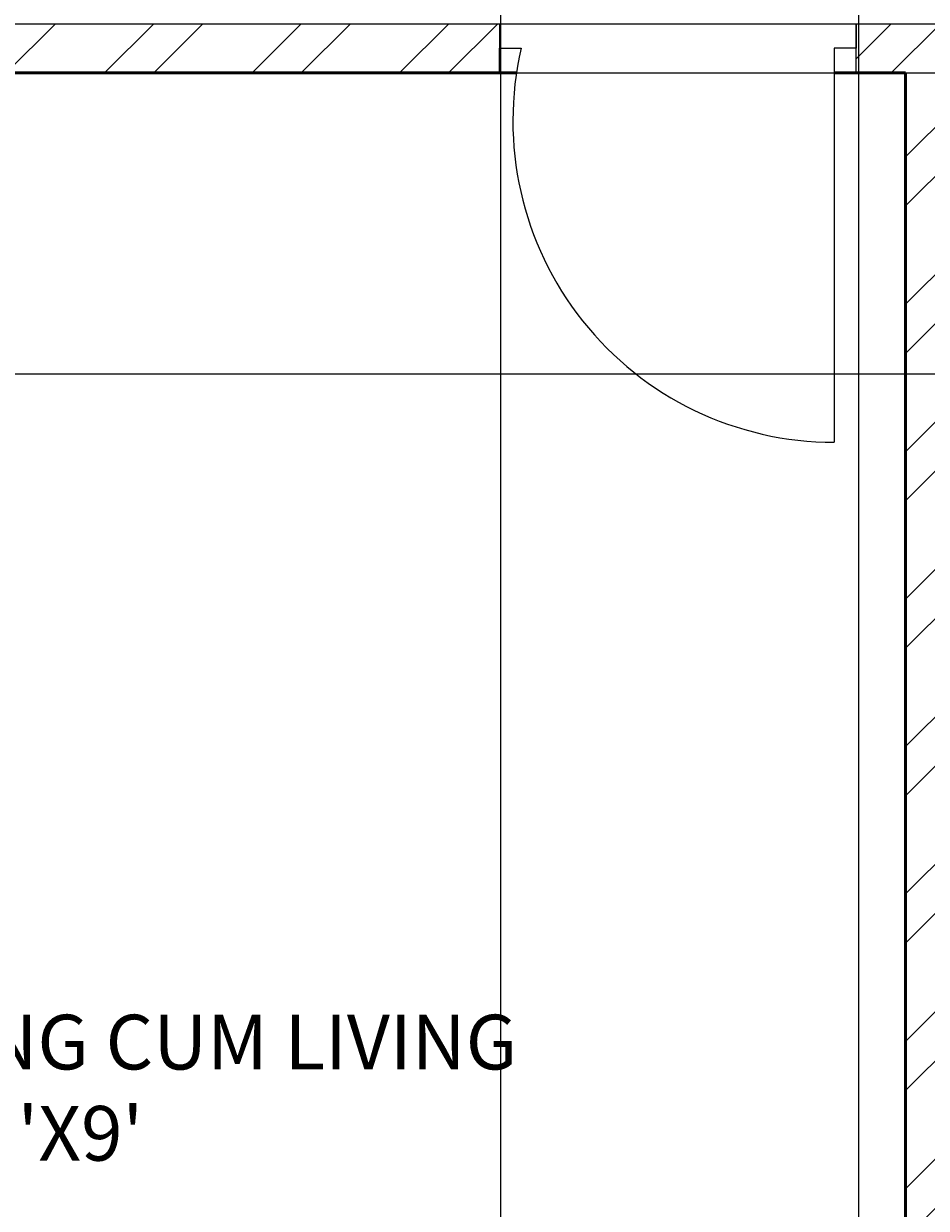
# Model space of a CAD drawing. Units: inches. Extents: x 2310 to 2937, y 1113 to 2410.
# Tile 7 of 23: x 2526 to 2609, y 1891 to 2000. Entities that reach past the tile are written whole.
import ezdxf

# ---------------------------------------------------------------- set-up
doc = ezdxf.new("R2010")
doc.units = ezdxf.units.IN
for name, color, linetype, lineweight in [('A-ANNO-DIMS', 2, 'Continuous', 18), ('A-AREA-IDEN', 7, 'Continuous', 18), ('A-DOOR', 31, 'Continuous', 25), ('A-WALL', 7, 'Continuous', 50), ('A-WALL-PATT', 85, 'Continuous', 13)]:
    doc.layers.add(name, color=color, linetype=linetype, lineweight=lineweight)
doc.styles.get("Standard").update_dxf_attribs({"font": 'arial.ttf'})
doc.dimstyles.get("Standard").update_dxf_attribs({"dimtxt": 0.18, "dimasz": 0.18, "dimexe": 0.18, "dimexo": 0.0625, "dimgap": 0.09, "dimtad": 0, "dimtih": 1, "dimtoh": 1, "dimdec": 4, "dimzin": 0, "dimdsep": 46, "dimtxsty": 'Standard', "dimcen": 0.09, "dimadec": 0, "dimazin": 0, "dimtfac": 1, "dimtdec": 4, "dimtofl": 0, "dimtmove": 0, "dimatfit": 3, "dimfxl": 1, "dimtolj": 1, "dimtzin": 0, "dimarcsym": 0})

# ---------------------------------------------------------------- blocks, each defined once
blk = doc.blocks.new('*D57')
at = {"layer": 'A-ANNO-DIMS', "color": 0, "lineweight": -2, "transparency": 16777216}
for p, q in [((2403.55, 1995.01), (2858.02, 1995.01)), ((2857.84, 1994.83), (2857.84, 1981.45)), ((2857.84, 1967.7), (2857.84, 1981.09)), ((2403.55, 1967.52), (2858.02, 1967.52))]:
    blk.add_line(p, q, dxfattribs=at)
at = {"layer": 'A-ANNO-DIMS', "color": 0, "transparency": 16777216}
for points in [[(2857.81, 1994.83), (2857.87, 1994.83), (2857.84, 1995.01)], [(2857.81, 1967.7), (2857.87, 1967.7), (2857.84, 1967.52)]]:
    blk.add_solid(points, dxfattribs=at)
at = {"layer": 'Defpoints', "color": 0, "transparency": 16777216}
for p in [(2403.49, 1995.01), (2403.49, 1967.52), (2857.84, 1967.52)]:
    blk.add_point(p, dxfattribs=at)
at = {"layer": 'A-ANNO-DIMS', "color": 0, "transparency": 16777216, "insert": (2857.84, 1981.27), "char_height": 0.18, "attachment_point": 5}
blk.add_mtext('\\A1;27.49', dxfattribs=at)
blk = doc.blocks.new('*D62')
at = {"layer": 'A-ANNO-DIMS', "color": 0, "lineweight": -2, "transparency": 16777216}
for p, q in [((2569.99, 2093.45), (2569.99, 1649.5)), ((2602.69, 2093.45), (2602.69, 1649.5)), ((2570.17, 1649.68), (2586.02, 1649.68)), ((2602.51, 1649.68), (2586.66, 1649.68))]:
    blk.add_line(p, q, dxfattribs=at)
at = {"layer": 'A-ANNO-DIMS', "color": 0, "transparency": 16777216}
for points in [[(2570.17, 1649.71), (2570.17, 1649.65), (2569.99, 1649.68)], [(2602.51, 1649.71), (2602.51, 1649.65), (2602.69, 1649.68)]]:
    blk.add_solid(points, dxfattribs=at)
at = {"layer": 'Defpoints', "color": 0, "transparency": 16777216}
for p in [(2569.99, 2093.51), (2602.69, 2093.51), (2602.69, 1649.68)]:
    blk.add_point(p, dxfattribs=at)
at = {"layer": 'A-ANNO-DIMS', "color": 0, "transparency": 16777216, "insert": (2586.34, 1649.68), "char_height": 0.18, "attachment_point": 5}
blk.add_mtext('\\A1;32.7', dxfattribs=at)
blk = doc.blocks.new('*D64')
at = {"layer": 'A-ANNO-DIMS', "color": 0, "lineweight": -2, "transparency": 16777216}
for p, q in [((2524.527191, 2046.513944), (2858.015941, 2046.513944)), ((2857.835941, 2046.333944), (2857.835941, 2023.193944)), ((2857.835941, 1999.693944), (2857.835941, 2022.833944)), ((2524.527191, 1999.513944), (2858.015941, 1999.513944))]:
    blk.add_line(p, q, dxfattribs=at)
at = {"layer": 'A-ANNO-DIMS', "color": 0, "transparency": 16777216}
for points in [[(2857.805941, 2046.333944), (2857.865941, 2046.333944), (2857.835941, 2046.513944)], [(2857.805941, 1999.693944), (2857.865941, 1999.693944), (2857.835941, 1999.513944)]]:
    blk.add_solid(points, dxfattribs=at)
at = {"layer": 'Defpoints', "color": 0, "transparency": 16777216}
for p in [(2524.464691, 2046.513944), (2857.835941, 2046.513944), (2524.464691, 1999.513944)]:
    blk.add_point(p, dxfattribs=at)
at = {"layer": 'A-ANNO-DIMS', "color": 0, "transparency": 16777216, "insert": (2857.835941, 2023.013944), "char_height": 0.18, "attachment_point": 5}
blk.add_mtext('\\A1;47', dxfattribs=at)

msp = doc.modelspace()

# ---------------------------------------------------------------- hatches: boundary and pattern name
at = {"layer": 'A-WALL-PATT'}
h = msp.add_hatch(dxfattribs=at)
h.set_pattern_fill('ANSI32', color=256)
h.paths.add_polyline_path([(2639.1394, 2356.5139), (2563.662, 2356.5139), (2563.662, 2347.5139), (2606.9859, 2347.5139), (2606.9859, 2210.5139), (2514.2692, 2210.5139), (2514.2692, 2206.0139), (2606.9859, 2206.0139), (2606.9859, 2098.0139), (2602.689, 2098.0139), (2602.689, 2093.5139), (2615.5262, 2093.5139), (2615.5262, 2095.7639), (2615.5262, 2098.0139), (2611.4859, 2098.0139), (2611.4859, 2206.0139), (2703.9391, 2206.0139), (2703.9391, 2208.2639), (2703.9391, 2210.5139), (2611.4859, 2210.5139), (2611.4859, 2347.5139), (2639.1394, 2347.5139)])
h.paths.add_polyline_path([(2823.9859, 2356.5139), (2699.1394, 2356.5139), (2699.1394, 2347.5139), (2738.4859, 2347.5139), (2738.4859, 2343.9266), (2742.9859, 2343.9266), (2742.9859, 2347.5139), (2814.9859, 2347.5139), (2814.9859, 2336.76), (2823.9859, 2336.76)])
h.paths.add_polyline_path([(2823.9859, 2312.76), (2814.9859, 2312.76), (2814.9859, 2299.5139), (2742.9859, 2299.5139), (2742.9859, 2323.0159), (2740.7359, 2323.0159), (2738.4859, 2323.0159), (2738.4859, 2210.5139), (2734.5483, 2210.5139), (2734.5483, 2206.0139), (2746.8769, 2206.0139), (2746.8769, 2208.2639), (2746.8769, 2210.5139), (2742.9859, 2210.5139), (2742.9859, 2295.0139), (2814.9859, 2295.0139), (2814.9859, 2269.8977), (2823.9859, 2269.8977)])
h.paths.add_polyline_path([(2823.9859, 2210.5139), (2823.9859, 2233.8977), (2819.4859, 2233.8977), (2814.9859, 2233.8977), (2814.9859, 2210.5139), (2769.9745, 2210.5139), (2769.9745, 2206.0139), (2814.9859, 2206.0139), (2814.9859, 2178.3027), (2823.9859, 2178.3027)])
h.paths.add_polyline_path([(2823.9859, 2118.3027), (2819.4859, 2118.3027), (2814.9859, 2118.3027), (2814.9859, 2098.0139), (2647.0333, 2098.0139), (2647.0333, 2093.5139), (2814.9859, 2093.5139), (2814.9859, 1999.5139), (2650.6052, 1999.5139), (2650.6052, 1995.0139), (2814.9859, 1995.0139), (2814.9859, 1969.9784), (2823.9859, 1969.9784)])
h.paths.add_polyline_path([(2403.4859, 2093.5139), (2569.9888, 2093.5139), (2569.9888, 2095.7639), (2569.9888, 2098.0139), (2403.4859, 2098.0139), (2403.4859, 2131.7587), (2394.4859, 2131.7587), (2394.4859, 1967.522), (2403.4859, 1967.522), (2403.4859, 1995.0139), (2569.8903, 1995.0139), (2569.8903, 1997.2639), (2569.8903, 1999.5139), (2403.4859, 1999.5139)])
h.paths.add_polyline_path([(2503.662, 2356.5139), (2394.4859, 2356.5139), (2394.4859, 2337.9231), (2398.9859, 2337.9231), (2403.4859, 2337.9231), (2403.4859, 2347.5139), (2475.4859, 2347.5139), (2475.4859, 2343.0384), (2479.9859, 2343.0384), (2479.9859, 2347.5139), (2503.662, 2347.5139)])
h.paths.add_polyline_path([(2498.3065, 1745.5139), (2479.9859, 1745.5139), (2479.9859, 1749.1663), (2477.7359, 1749.1663), (2475.4859, 1749.1663), (2475.4859, 1745.5139), (2403.4859, 1745.5139), (2403.4859, 1753.6409), (2398.9859, 1753.6409), (2394.4859, 1753.6409), (2394.4859, 1736.5139), (2498.3065, 1736.5139), (2498.3065, 1741.0139)])
h.paths.add_polyline_path([(2479.9859, 1882.5139), (2483.9367, 1882.5139), (2483.9367, 1887.0139), (2471.5501, 1887.0139), (2471.5501, 1885.1969), (2471.5501, 1882.5139), (2475.4859, 1882.5139), (2475.4859, 1798.0139), (2403.4859, 1798.0139), (2403.4859, 1828.0433), (2402.2852, 1828.0433), (2394.4859, 1828.0433), (2394.4859, 1777.6409), (2403.4859, 1777.6409), (2403.4859, 1793.5139), (2475.4859, 1793.5139), (2475.4859, 1769.1696), (2479.9859, 1769.1696)])
h.paths.add_polyline_path([(2403.4859, 1907.522), (2398.9859, 1907.522), (2394.4859, 1907.522), (2394.4859, 1864.0433), (2403.4859, 1864.0433), (2403.4859, 1882.5139), (2448.9325, 1882.5139), (2448.9325, 1884.7639), (2448.9325, 1887.0139), (2403.4859, 1887.0139)])
h.paths.add_polyline_path([(2702.2061, 1887.0139), (2611.4859, 1887.0139), (2611.4859, 1995.0139), (2615.6132, 1995.0139), (2615.6132, 1999.5139), (2602.4798, 1999.5139), (2602.4798, 1997.2639), (2602.4798, 1995.0139), (2606.9859, 1995.0139), (2606.9859, 1887.0139), (2516.2443, 1887.0139), (2516.2443, 1884.7639), (2516.2443, 1882.5139), (2606.9859, 1882.5139), (2606.9859, 1745.5139), (2558.3065, 1745.5139), (2558.3065, 1736.5139), (2638.8921, 1736.5139), (2638.8921, 1741.0139), (2638.8921, 1745.5139), (2611.4859, 1745.5139), (2611.4859, 1882.5139), (2702.2061, 1882.5139)])
h.paths.add_polyline_path([(2823.9859, 1909.9784), (2819.4859, 1909.9784), (2814.9859, 1909.9784), (2814.9859, 1887.0139), (2769.144, 1887.0139), (2769.144, 1884.7639), (2769.144, 1882.5139), (2814.9859, 1882.5139), (2814.9859, 1854.1704), (2823.9859, 1854.1704)])
h.paths.add_polyline_path([(2823.9859, 1818.1704), (2819.4859, 1818.1704), (2814.9859, 1818.1704), (2814.9859, 1798.0139), (2742.9859, 1798.0139), (2742.9859, 1882.5139), (2746.805, 1882.5139), (2746.805, 1887.0139), (2733.7334, 1887.0139), (2733.7334, 1884.7639), (2733.7334, 1882.5139), (2738.4859, 1882.5139), (2738.4859, 1771.1728), (2740.7359, 1771.1728), (2742.9859, 1771.1728), (2742.9859, 1793.5139), (2814.9859, 1793.5139), (2814.9859, 1783.6684), (2823.9859, 1783.6684)])
h.paths.add_polyline_path([(2823.9859, 1759.6684), (2814.9859, 1759.6684), (2814.9859, 1745.5139), (2742.9859, 1745.5139), (2742.9859, 1748.9831), (2740.7359, 1748.9831), (2738.4859, 1748.9831), (2738.4859, 1745.5139), (2698.8921, 1745.5139), (2698.8921, 1736.5139), (2823.9859, 1736.5139)])

# ---------------------------------------------------------------- linework, layer by layer
at = {"layer": 'A-DOOR'}
for p, q in [((2569.8903, 1999.5139), (2569.8903, 1995.0139)), ((2602.4798, 1995.0139), (2602.4798, 1999.5139)), ((2602.4798, 1999.5139), (2602.4798, 1997.2639)), ((2569.8903, 1995.0139), (2569.8903, 1997.2639)), ((2569.8903, 1997.2639), (2571.8903, 1997.2639)), ((2602.4798, 1997.2639), (2600.4798, 1997.2639)), ((2600.4798, 1997.2639), (2600.4798, 1961.2639))]:
    msp.add_line(p, q, dxfattribs=at)
msp.add_arc((2600.4798, 1990.6162), 29.3523, 166.909972, 270, dxfattribs=at)
at = {"layer": 'A-WALL'}
for p, q in [((2403.4859, 1995.0139), (2571.4589, 1995.0139)), ((2600.4798, 1995.0139), (2606.9859, 1995.0139)), ((2606.9859, 1995.0139), (2606.9859, 1887.0139))]:
    msp.add_line(p, q, dxfattribs=at)

# ---------------------------------------------------------------- texts
at = {"layer": 'A-AREA-IDEN', "insert": (2495.3926, 1908.9628), "char_height": 5, "attachment_point": 1}
msp.add_mtext_dynamic_manual_height_columns("         DINING CUM LIVING\\P               17'X9'", width=186.629206, gutter_width=12.5, heights=[0], dxfattribs=at)

# ---------------------------------------------------------------- dimensions: what is measured, and where the dimension line sits
at = {"layer": 'A-ANNO-DIMS'}
dim = msp.add_linear_dim(base=(2602.689, 1649.6807), p1=(2569.9888, 2093.5139), p2=(2602.689, 2093.5139), dimstyle='Standard', override={"dimdec": 1, "dimlfac": 1, "dimrnd": 0, "dimzin": 0, "dimdsep": 46, "dimlunit": 2}, dxfattribs=at)
dim.commit()
dim.dimension.update_dxf_attribs({"geometry": '*D62', "text_midpoint": (2586.3389, 1649.6807)})
for base, p1, p2, override, picture, middle in [((2857.8359, 2046.5139), (2524.4647, 1999.5139), (2524.4647, 2046.5139), {"dimdec": 0, "dimlfac": 1, "dimrnd": 0, "dimzin": 0, "dimdsep": 46, "dimlunit": 2}, '*D64', (2857.8359, 2023.0139)), ((2857.8359, 1967.522), (2403.4859, 1995.0139), (2403.4859, 1967.522), {"dimdec": 2, "dimlfac": 1, "dimrnd": 0, "dimzin": 0, "dimdsep": 46, "dimlunit": 2}, '*D57', (2857.8359, 1981.268))]:
    dim = msp.add_linear_dim(base=base, p1=p1, p2=p2, angle=90, dimstyle='Standard', override=override, dxfattribs=at)
    dim.commit()
    dim.dimension.update_dxf_attribs({"geometry": picture, "text_midpoint": middle})

doc.saveas('drawing.dxf')
